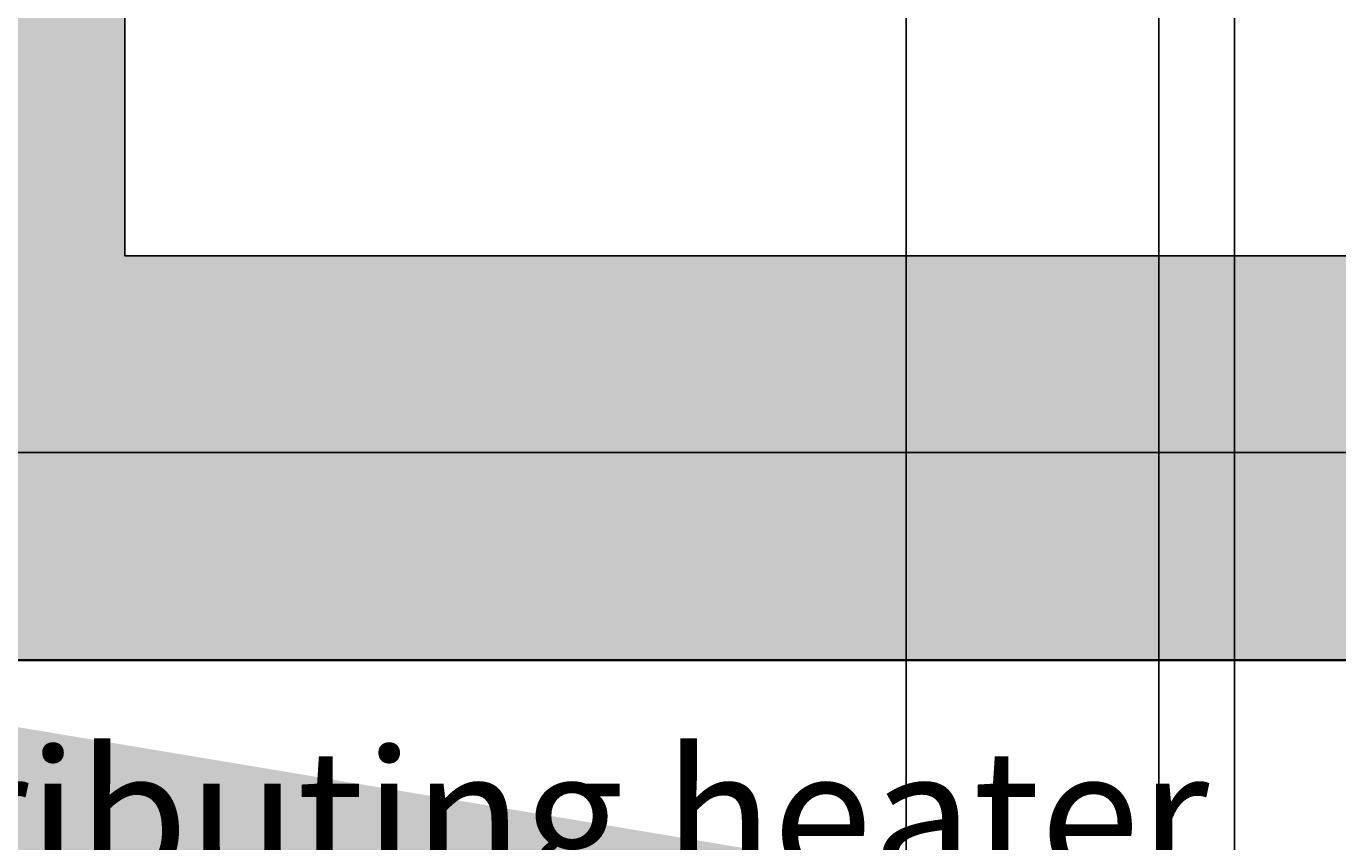
# Model space of a CAD drawing. Units: millimetres. Extents: x -22994 to 29398, y -19990 to 20176.
# Tile 27 of 135: x 99 to 139, y 5 to 30. Entities that reach past the tile are written whole.
import ezdxf
from ezdxf import colors
from ezdxf.entities.mleader import LeaderData, LeaderLine
from ezdxf.math import Vec2, Vec3

# ---------------------------------------------------------------- set-up
doc = ezdxf.new("R2010")
doc.units = ezdxf.units.MM
doc.header["$MEASUREMENT"] = 0
for name, color, linetype, lineweight in [('M-ANNO-TEXT', 7, 'Continuous', 25), ('M-DIMS', 2, 'Continuous', 18), ('M-EQPM', 7, 'Continuous', 25), ('M-EQPM-PATT', 7, 'Continuous', 18), ('S-FNDN', 7, 'Continuous', 35)]:
    doc.layers.add(name, color=color, linetype=linetype, lineweight=lineweight)
doc.styles.get("Standard").update_dxf_attribs({"font": 'arial.ttf'})
doc.dimstyles.get("Standard").update_dxf_attribs({"dimtxt": 0.18, "dimasz": 10000, "dimexe": 0.18, "dimexo": 0.0625, "dimgap": 0.09, "dimtad": 0, "dimtih": 1, "dimtoh": 1, "dimdec": 0, "dimzin": 0, "dimdsep": 46, "dimtxsty": 'Standard', "dimcen": 0.09, "dimadec": 0, "dimazin": 0, "dimtfac": 1, "dimtdec": 0, "dimtofl": 0, "dimtmove": 0, "dimatfit": 3, "dimfxl": 1, "dimtolj": 1, "dimtzin": 0, "dimlwd": 30, "dimarcsym": 0})

# ---------------------------------------------------------------- blocks, each defined once
blk = doc.blocks.new('*D2')
at = {"layer": 'Defpoints', "color": 0, "transparency": 16777216}
for p in [(6.677, 10.271), (290.852, 10.271), (290.852, -5.079)]:
    blk.add_point(p, dxfattribs=at)
at = {"layer": 'M-DIMS', "color": 0, "lineweight": -2, "transparency": 16777216}
for p, q in [((6.677, 10.209), (6.677, -5.259)), ((290.852, 10.209), (290.852, -5.259))]:
    blk.add_line(p, q, dxfattribs=at)
at = {"layer": 'M-DIMS', "color": 0, "lineweight": 30, "transparency": 16777216}
for p, q in [((-9993.323, -5.079), (-19993.323, -5.079)), ((10290.852, -5.079), (20290.852, -5.079))]:
    blk.add_line(p, q, dxfattribs=at)
at = {"layer": 'M-DIMS', "color": 0, "transparency": 16777216}
for points in [[(-9993.323, 1661.588), (-9993.323, -1671.745), (6.677, -5.079)], [(10290.852, 1661.588), (10290.852, -1671.745), (290.852, -5.079)]]:
    blk.add_solid(points, dxfattribs=at)
at = {"layer": 'M-DIMS', "color": 0, "transparency": 16777216, "insert": (148.765, -5.079), "char_height": 0.18, "attachment_point": 5}
blk.add_mtext('\\A1;284.2', dxfattribs=at)
blk = doc.blocks.new('*D3')
at = {"layer": 'Defpoints', "color": 0, "transparency": 16777216}
for p in [(110.265, 204.165), (110.265, 176.366), (95.833, 127.967)]:
    blk.add_point(p, dxfattribs=at)
at = {"layer": 'M-DIMS', "color": 0, "lineweight": -2, "transparency": 16777216}
for p, q in [((95.833, 128.03), (95.833, 204.345)), ((110.265, 176.429), (110.265, 204.345))]:
    blk.add_line(p, q, dxfattribs=at)
at = {"layer": 'M-DIMS', "color": 0, "lineweight": 30, "transparency": 16777216}
for p, q in [((-9904.167, 204.165), (-19904.167, 204.165)), ((10110.265, 204.165), (20110.265, 204.165))]:
    blk.add_line(p, q, dxfattribs=at)
at = {"layer": 'M-DIMS', "color": 0, "transparency": 16777216}
for points in [[(-9904.167, 1870.832), (-9904.167, -1462.501), (95.833, 204.165)], [(10110.265, 1870.832), (10110.265, -1462.501), (110.265, 204.165)]]:
    blk.add_solid(points, dxfattribs=at)
at = {"layer": 'M-DIMS', "color": 0, "transparency": 16777216, "insert": (103.049, 204.165), "char_height": 0.18, "attachment_point": 5}
blk.add_mtext('\\A1;14.432', dxfattribs=at)
blk = doc.blocks.new('*D4')
at = {"layer": 'Defpoints', "color": 0, "transparency": 16777216}
for p in [(116.265, 204.165), (110.265, 176.366), (116.265, 176.366)]:
    blk.add_point(p, dxfattribs=at)
at = {"layer": 'M-DIMS', "color": 0, "lineweight": -2, "transparency": 16777216}
for p, q in [((110.265, 176.429), (110.265, 204.345)), ((116.265, 176.429), (116.265, 204.345))]:
    blk.add_line(p, q, dxfattribs=at)
at = {"layer": 'M-DIMS', "color": 0, "lineweight": 30, "transparency": 16777216}
for p, q in [((-9889.735, 204.165), (-19889.735, 204.165)), ((10116.265, 204.165), (20116.265, 204.165))]:
    blk.add_line(p, q, dxfattribs=at)
at = {"layer": 'M-DIMS', "color": 0, "transparency": 16777216}
for points in [[(-9889.735, 1870.832), (-9889.735, -1462.501), (110.265, 204.165)], [(10116.265, 1870.832), (10116.265, -1462.501), (116.265, 204.165)]]:
    blk.add_solid(points, dxfattribs=at)
at = {"layer": 'M-DIMS', "color": 0, "transparency": 16777216, "insert": (113.265, 204.165), "char_height": 0.18, "attachment_point": 5}
blk.add_mtext('\\A1;6', dxfattribs=at)
blk = doc.blocks.new('*D5')
at = {"layer": 'Defpoints', "color": 0, "transparency": 16777216}
for p in [(181.265, 204.165), (116.265, 176.366), (181.265, 176.366)]:
    blk.add_point(p, dxfattribs=at)
at = {"layer": 'M-DIMS', "color": 0, "lineweight": -2, "transparency": 16777216}
for p, q in [((116.265, 176.429), (116.265, 204.345)), ((181.265, 176.429), (181.265, 204.345))]:
    blk.add_line(p, q, dxfattribs=at)
at = {"layer": 'M-DIMS', "color": 0, "lineweight": 30, "transparency": 16777216}
for p, q in [((-9883.735, 204.165), (-19883.735, 204.165)), ((10181.265, 204.165), (20181.265, 204.165))]:
    blk.add_line(p, q, dxfattribs=at)
at = {"layer": 'M-DIMS', "color": 0, "transparency": 16777216}
for points in [[(-9883.735, 1870.832), (-9883.735, -1462.501), (116.265, 204.165)], [(10181.265, 1870.832), (10181.265, -1462.501), (181.265, 204.165)]]:
    blk.add_solid(points, dxfattribs=at)
at = {"layer": 'M-DIMS', "color": 0, "transparency": 16777216, "insert": (148.765, 204.165), "char_height": 0.18, "attachment_point": 5}
blk.add_mtext('\\A1;65', dxfattribs=at)
blk = doc.blocks.new('*D6')
at = {"layer": 'Defpoints', "color": 0, "transparency": 16777216}
for p in [(187.265, 204.165), (181.265, 176.366), (187.265, 176.366)]:
    blk.add_point(p, dxfattribs=at)
at = {"layer": 'M-DIMS', "color": 0, "lineweight": -2, "transparency": 16777216}
for p, q in [((181.265, 176.429), (181.265, 204.345)), ((187.265, 176.429), (187.265, 204.345))]:
    blk.add_line(p, q, dxfattribs=at)
at = {"layer": 'M-DIMS', "color": 0, "lineweight": 30, "transparency": 16777216}
for p, q in [((-9818.735, 204.165), (-19818.735, 204.165)), ((10187.265, 204.165), (20187.265, 204.165))]:
    blk.add_line(p, q, dxfattribs=at)
at = {"layer": 'M-DIMS', "color": 0, "transparency": 16777216}
for points in [[(-9818.735, 1870.832), (-9818.735, -1462.501), (181.265, 204.165)], [(10187.265, 1870.832), (10187.265, -1462.501), (187.265, 204.165)]]:
    blk.add_solid(points, dxfattribs=at)
at = {"layer": 'M-DIMS', "color": 0, "transparency": 16777216, "insert": (184.265, 204.165), "char_height": 0.18, "attachment_point": 5}
blk.add_mtext('\\A1;6', dxfattribs=at)
blk = doc.blocks.new('*D7')
at = {"layer": 'Defpoints', "color": 0, "transparency": 16777216}
for p in [(201.697, 204.165), (187.265, 176.366), (201.697, 127.967)]:
    blk.add_point(p, dxfattribs=at)
at = {"layer": 'M-DIMS', "color": 0, "lineweight": -2, "transparency": 16777216}
for p, q in [((187.265, 176.429), (187.265, 204.345)), ((201.697, 128.03), (201.697, 204.345))]:
    blk.add_line(p, q, dxfattribs=at)
at = {"layer": 'M-DIMS', "color": 0, "lineweight": 30, "transparency": 16777216}
for p, q in [((-9812.735, 204.165), (-19812.735, 204.165)), ((10201.697, 204.165), (20201.697, 204.165))]:
    blk.add_line(p, q, dxfattribs=at)
at = {"layer": 'M-DIMS', "color": 0, "transparency": 16777216}
for points in [[(-9812.735, 1870.832), (-9812.735, -1462.501), (187.265, 204.165)], [(10201.697, 1870.832), (10201.697, -1462.501), (201.697, 204.165)]]:
    blk.add_solid(points, dxfattribs=at)
at = {"layer": 'M-DIMS', "color": 0, "transparency": 16777216, "insert": (194.481, 204.165), "char_height": 0.18, "attachment_point": 5}
blk.add_mtext('\\A1;14.432', dxfattribs=at)
blk = doc.blocks.new('*D8')
at = {"layer": 'Defpoints', "color": 0, "transparency": 16777216}
for p in [(227.648, 204.165), (227.648, 146.73), (201.697, 127.967)]:
    blk.add_point(p, dxfattribs=at)
at = {"layer": 'M-DIMS', "color": 0, "lineweight": -2, "transparency": 16777216}
for p, q in [((201.697, 128.03), (201.697, 204.345)), ((227.648, 146.792), (227.648, 204.345))]:
    blk.add_line(p, q, dxfattribs=at)
at = {"layer": 'M-DIMS', "color": 0, "lineweight": 30, "transparency": 16777216}
for p, q in [((-9798.303, 204.165), (-19798.303, 204.165)), ((10227.648, 204.165), (20227.648, 204.165))]:
    blk.add_line(p, q, dxfattribs=at)
at = {"layer": 'M-DIMS', "color": 0, "transparency": 16777216}
for points in [[(-9798.303, 1870.832), (-9798.303, -1462.501), (201.697, 204.165)], [(10227.648, 1870.832), (10227.648, -1462.501), (227.648, 204.165)]]:
    blk.add_solid(points, dxfattribs=at)
at = {"layer": 'M-DIMS', "color": 0, "transparency": 16777216, "insert": (214.673, 204.165), "char_height": 0.18, "attachment_point": 5}
blk.add_mtext('\\A1;25.95', dxfattribs=at)
blk = doc.blocks.new('*D9')
at = {"layer": 'Defpoints', "color": 0, "transparency": 16777216}
for p in [(187.265, 176.366), (306.202, 176.366), (290.852, 10.271)]:
    blk.add_point(p, dxfattribs=at)
at = {"layer": 'M-DIMS', "color": 0, "lineweight": 30, "transparency": 16777216}
for p, q in [((306.202, 10176.366), (306.202, 20176.366)), ((306.202, -9989.729), (306.202, -19989.729))]:
    blk.add_line(p, q, dxfattribs=at)
at = {"layer": 'M-DIMS', "color": 0, "lineweight": -2, "transparency": 16777216}
for p, q in [((187.327, 176.366), (306.382, 176.366)), ((290.915, 10.271), (306.382, 10.271))]:
    blk.add_line(p, q, dxfattribs=at)
at = {"layer": 'M-DIMS', "color": 0, "transparency": 16777216}
for points in [[(-1360.465, 10176.366), (1972.869, 10176.366), (306.202, 176.366)], [(-1360.465, -9989.729), (1972.869, -9989.729), (306.202, 10.271)]]:
    blk.add_solid(points, dxfattribs=at)
at = {"layer": 'M-DIMS', "color": 0, "transparency": 16777216, "insert": (306.202, 93.319), "char_height": 0.18, "attachment_point": 5}
blk.add_mtext('\\A1;166.1', dxfattribs=at)
blk = doc.blocks.new('*D10')
at = {"layer": 'Defpoints', "color": 0, "transparency": 16777216}
for p in [(125.65, 136.071), (133.346, 136.071), (133.346, -5.079)]:
    blk.add_point(p, dxfattribs=at)
at = {"layer": 'M-DIMS', "color": 0, "lineweight": -2, "transparency": 16777216}
for p, q in [((125.65, 136.009), (125.65, -5.259)), ((133.346, 136.009), (133.346, -5.259))]:
    blk.add_line(p, q, dxfattribs=at)
at = {"layer": 'M-DIMS', "color": 0, "lineweight": 30, "transparency": 16777216}
for p, q in [((-9874.35, -5.079), (-19874.35, -5.079)), ((10133.346, -5.079), (20133.346, -5.079))]:
    blk.add_line(p, q, dxfattribs=at)
at = {"layer": 'M-DIMS', "color": 0, "transparency": 16777216}
for points in [[(-9874.35, 1661.588), (-9874.35, -1671.745), (125.65, -5.079)], [(10133.346, 1661.588), (10133.346, -1671.745), (133.346, -5.079)]]:
    blk.add_solid(points, dxfattribs=at)
at = {"layer": 'M-DIMS', "color": 0, "transparency": 16777216, "insert": (129.498, -5.079), "char_height": 0.18, "attachment_point": 5}
blk.add_mtext('\\A1;7.696', dxfattribs=at)
blk = doc.blocks.new('*D11')
at = {"layer": 'Defpoints', "color": 0, "transparency": 16777216}
for p in [(133.346, 136.071), (135.65, 136.071), (135.65, -5.079)]:
    blk.add_point(p, dxfattribs=at)
at = {"layer": 'M-DIMS', "color": 0, "lineweight": -2, "transparency": 16777216}
for p, q in [((133.346, 136.009), (133.346, -5.259)), ((135.65, 136.009), (135.65, -5.259))]:
    blk.add_line(p, q, dxfattribs=at)
at = {"layer": 'M-DIMS', "color": 0, "lineweight": 30, "transparency": 16777216}
for p, q in [((-9866.654, -5.079), (-19866.654, -5.079)), ((10135.65, -5.079), (20135.65, -5.079))]:
    blk.add_line(p, q, dxfattribs=at)
at = {"layer": 'M-DIMS', "color": 0, "transparency": 16777216}
for points in [[(-9866.654, 1661.588), (-9866.654, -1671.745), (133.346, -5.079)], [(10135.65, 1661.588), (10135.65, -1671.745), (135.65, -5.079)]]:
    blk.add_solid(points, dxfattribs=at)
at = {"layer": 'M-DIMS', "color": 0, "transparency": 16777216, "insert": (134.498, -5.079), "char_height": 0.18, "attachment_point": 5}
blk.add_mtext('\\A1;2.304', dxfattribs=at)
blk = doc.blocks.new('*D12')
at = {"layer": 'Defpoints', "color": 0, "transparency": 16777216}
for p in [(135.65, 136.071), (145.65, 136.071), (145.65, -5.079)]:
    blk.add_point(p, dxfattribs=at)
at = {"layer": 'M-DIMS', "color": 0, "lineweight": -2, "transparency": 16777216}
for p, q in [((135.65, 136.009), (135.65, -5.259)), ((145.65, 136.009), (145.65, -5.259))]:
    blk.add_line(p, q, dxfattribs=at)
at = {"layer": 'M-DIMS', "color": 0, "lineweight": 30, "transparency": 16777216}
for p, q in [((-9864.35, -5.079), (-19864.35, -5.079)), ((10145.65, -5.079), (20145.65, -5.079))]:
    blk.add_line(p, q, dxfattribs=at)
at = {"layer": 'M-DIMS', "color": 0, "transparency": 16777216}
for points in [[(-9864.35, 1661.588), (-9864.35, -1671.745), (135.65, -5.079)], [(10145.65, 1661.588), (10145.65, -1671.745), (145.65, -5.079)]]:
    blk.add_solid(points, dxfattribs=at)
at = {"layer": 'M-DIMS', "color": 0, "transparency": 16777216, "insert": (140.65, -5.079), "char_height": 0.18, "attachment_point": 5}
blk.add_mtext('\\A1;10', dxfattribs=at)
blk = doc.blocks.new('*D13')
at = {"layer": 'Defpoints', "color": 0, "transparency": 16777216}
for p in [(145.65, 136.071), (155.65, 136.071), (155.65, -5.079)]:
    blk.add_point(p, dxfattribs=at)
at = {"layer": 'M-DIMS', "color": 0, "lineweight": -2, "transparency": 16777216}
for p, q in [((145.65, 136.009), (145.65, -5.259)), ((155.65, 136.009), (155.65, -5.259))]:
    blk.add_line(p, q, dxfattribs=at)
at = {"layer": 'M-DIMS', "color": 0, "lineweight": 30, "transparency": 16777216}
for p, q in [((-9854.35, -5.079), (-19854.35, -5.079)), ((10155.65, -5.079), (20155.65, -5.079))]:
    blk.add_line(p, q, dxfattribs=at)
at = {"layer": 'M-DIMS', "color": 0, "transparency": 16777216}
for points in [[(-9854.35, 1661.588), (-9854.35, -1671.745), (145.65, -5.079)], [(10155.65, 1661.588), (10155.65, -1671.745), (155.65, -5.079)]]:
    blk.add_solid(points, dxfattribs=at)
at = {"layer": 'M-DIMS', "color": 0, "transparency": 16777216, "insert": (150.65, -5.079), "char_height": 0.18, "attachment_point": 5}
blk.add_mtext('\\A1;10', dxfattribs=at)
blk = doc.blocks.new('*D14')
at = {"layer": 'Defpoints', "color": 0, "transparency": 16777216}
for p in [(155.65, 136.071), (165.65, 136.071), (165.65, -5.079)]:
    blk.add_point(p, dxfattribs=at)
at = {"layer": 'M-DIMS', "color": 0, "lineweight": -2, "transparency": 16777216}
for p, q in [((155.65, 136.009), (155.65, -5.259)), ((165.65, 136.009), (165.65, -5.259))]:
    blk.add_line(p, q, dxfattribs=at)
at = {"layer": 'M-DIMS', "color": 0, "lineweight": 30, "transparency": 16777216}
for p, q in [((-9844.35, -5.079), (-19844.35, -5.079)), ((10165.65, -5.079), (20165.65, -5.079))]:
    blk.add_line(p, q, dxfattribs=at)
at = {"layer": 'M-DIMS', "color": 0, "transparency": 16777216}
for points in [[(-9844.35, 1661.588), (-9844.35, -1671.745), (155.65, -5.079)], [(10165.65, 1661.588), (10165.65, -1671.745), (165.65, -5.079)]]:
    blk.add_solid(points, dxfattribs=at)
at = {"layer": 'M-DIMS', "color": 0, "transparency": 16777216, "insert": (160.65, -5.079), "char_height": 0.18, "attachment_point": 5}
blk.add_mtext('\\A1;10', dxfattribs=at)
blk = doc.blocks.new('*D15')
at = {"layer": 'Defpoints', "color": 0, "transparency": 16777216}
for p in [(173.346, 154.788), (173.346, 136.071), (306.202, 136.071)]:
    blk.add_point(p, dxfattribs=at)
at = {"layer": 'M-DIMS', "color": 0, "lineweight": 30, "transparency": 16777216}
for p, q in [((306.202, 10154.788), (306.202, 20154.788)), ((306.202, -9863.929), (306.202, -19863.929))]:
    blk.add_line(p, q, dxfattribs=at)
at = {"layer": 'M-DIMS', "color": 0, "lineweight": -2, "transparency": 16777216}
for p, q in [((173.408, 154.788), (306.382, 154.788)), ((173.408, 136.071), (306.382, 136.071))]:
    blk.add_line(p, q, dxfattribs=at)
at = {"layer": 'M-DIMS', "color": 0, "transparency": 16777216}
for points in [[(-1360.465, 10154.788), (1972.869, 10154.788), (306.202, 154.788)], [(-1360.465, -9863.929), (1972.869, -9863.929), (306.202, 136.071)]]:
    blk.add_solid(points, dxfattribs=at)
at = {"layer": 'M-DIMS', "color": 0, "transparency": 16777216, "insert": (306.202, 145.43), "char_height": 0.18, "attachment_point": 5}
blk.add_mtext('\\A1;18.717', dxfattribs=at)
blk = doc.blocks.new('*D16')
at = {"layer": 'Defpoints', "color": 0, "transparency": 16777216}
for p in [(120.17, 204.165), (110.466, 48.035), (120.17, 48.035)]:
    blk.add_point(p, dxfattribs=at)
at = {"layer": 'M-DIMS', "color": 0, "lineweight": -2, "transparency": 16777216}
for p, q in [((110.466, 48.097), (110.466, 204.345)), ((120.17, 48.097), (120.17, 204.345))]:
    blk.add_line(p, q, dxfattribs=at)
at = {"layer": 'M-DIMS', "color": 0, "lineweight": 30, "transparency": 16777216}
for p, q in [((-9889.534, 204.165), (-19889.534, 204.165)), ((10120.17, 204.165), (20120.17, 204.165))]:
    blk.add_line(p, q, dxfattribs=at)
at = {"layer": 'M-DIMS', "color": 0, "transparency": 16777216}
for points in [[(-9889.534, 1870.832), (-9889.534, -1462.501), (110.466, 204.165)], [(10120.17, 1870.832), (10120.17, -1462.501), (120.17, 204.165)]]:
    blk.add_solid(points, dxfattribs=at)
at = {"layer": 'M-DIMS', "color": 0, "transparency": 16777216, "insert": (115.318, 204.165), "char_height": 0.18, "attachment_point": 5}
blk.add_mtext('\\A1;9.704', dxfattribs=at)
blk = doc.blocks.new('*D17')
at = {"layer": 'Defpoints', "color": 0, "transparency": 16777216}
for p in [(126.17, 204.165), (120.17, 48.035), (126.17, 48.035)]:
    blk.add_point(p, dxfattribs=at)
at = {"layer": 'M-DIMS', "color": 0, "lineweight": -2, "transparency": 16777216}
for p, q in [((120.17, 48.097), (120.17, 204.345)), ((126.17, 48.097), (126.17, 204.345))]:
    blk.add_line(p, q, dxfattribs=at)
at = {"layer": 'M-DIMS', "color": 0, "lineweight": 30, "transparency": 16777216}
for p, q in [((-9879.83, 204.165), (-19879.83, 204.165)), ((10126.17, 204.165), (20126.17, 204.165))]:
    blk.add_line(p, q, dxfattribs=at)
at = {"layer": 'M-DIMS', "color": 0, "transparency": 16777216}
for points in [[(-9879.83, 1870.832), (-9879.83, -1462.501), (120.17, 204.165)], [(10126.17, 1870.832), (10126.17, -1462.501), (126.17, 204.165)]]:
    blk.add_solid(points, dxfattribs=at)
at = {"layer": 'M-DIMS', "color": 0, "transparency": 16777216, "insert": (123.17, 204.165), "char_height": 0.18, "attachment_point": 5}
blk.add_mtext('\\A1;6', dxfattribs=at)
blk = doc.blocks.new('*D18')
at = {"layer": 'Defpoints', "color": 0, "transparency": 16777216}
for p in [(132.17, 204.165), (126.17, 48.035), (132.17, 48.035)]:
    blk.add_point(p, dxfattribs=at)
at = {"layer": 'M-DIMS', "color": 0, "lineweight": -2, "transparency": 16777216}
for p, q in [((126.17, 48.097), (126.17, 204.345)), ((132.17, 48.097), (132.17, 204.345))]:
    blk.add_line(p, q, dxfattribs=at)
at = {"layer": 'M-DIMS', "color": 0, "lineweight": 30, "transparency": 16777216}
for p, q in [((-9873.83, 204.165), (-19873.83, 204.165)), ((10132.17, 204.165), (20132.17, 204.165))]:
    blk.add_line(p, q, dxfattribs=at)
at = {"layer": 'M-DIMS', "color": 0, "transparency": 16777216}
for points in [[(-9873.83, 1870.832), (-9873.83, -1462.501), (126.17, 204.165)], [(10132.17, 1870.832), (10132.17, -1462.501), (132.17, 204.165)]]:
    blk.add_solid(points, dxfattribs=at)
at = {"layer": 'M-DIMS', "color": 0, "transparency": 16777216, "insert": (129.17, 204.165), "char_height": 0.18, "attachment_point": 5}
blk.add_mtext('\\A1;6', dxfattribs=at)
blk = doc.blocks.new('*D19')
at = {"layer": 'Defpoints', "color": 0, "transparency": 16777216}
for p in [(138.17, 204.165), (132.17, 48.035), (138.17, 48.035)]:
    blk.add_point(p, dxfattribs=at)
at = {"layer": 'M-DIMS', "color": 0, "lineweight": -2, "transparency": 16777216}
for p, q in [((132.17, 48.097), (132.17, 204.345)), ((138.17, 48.097), (138.17, 204.345))]:
    blk.add_line(p, q, dxfattribs=at)
at = {"layer": 'M-DIMS', "color": 0, "lineweight": 30, "transparency": 16777216}
for p, q in [((-9867.83, 204.165), (-19867.83, 204.165)), ((10138.17, 204.165), (20138.17, 204.165))]:
    blk.add_line(p, q, dxfattribs=at)
at = {"layer": 'M-DIMS', "color": 0, "transparency": 16777216}
for points in [[(-9867.83, 1870.832), (-9867.83, -1462.501), (132.17, 204.165)], [(10138.17, 1870.832), (10138.17, -1462.501), (138.17, 204.165)]]:
    blk.add_solid(points, dxfattribs=at)
at = {"layer": 'M-DIMS', "color": 0, "transparency": 16777216, "insert": (135.17, 204.165), "char_height": 0.18, "attachment_point": 5}
blk.add_mtext('\\A1;6', dxfattribs=at)
blk = doc.blocks.new('*D20')
at = {"layer": 'Defpoints', "color": 0, "transparency": 16777216}
for p in [(144.17, 204.165), (138.17, 48.035), (144.17, 48.035)]:
    blk.add_point(p, dxfattribs=at)
at = {"layer": 'M-DIMS', "color": 0, "lineweight": -2, "transparency": 16777216}
for p, q in [((138.17, 48.097), (138.17, 204.345)), ((144.17, 48.097), (144.17, 204.345))]:
    blk.add_line(p, q, dxfattribs=at)
at = {"layer": 'M-DIMS', "color": 0, "lineweight": 30, "transparency": 16777216}
for p, q in [((-9861.83, 204.165), (-19861.83, 204.165)), ((10144.17, 204.165), (20144.17, 204.165))]:
    blk.add_line(p, q, dxfattribs=at)
at = {"layer": 'M-DIMS', "color": 0, "transparency": 16777216}
for points in [[(-9861.83, 1870.832), (-9861.83, -1462.501), (138.17, 204.165)], [(10144.17, 1870.832), (10144.17, -1462.501), (144.17, 204.165)]]:
    blk.add_solid(points, dxfattribs=at)
at = {"layer": 'M-DIMS', "color": 0, "transparency": 16777216, "insert": (141.17, 204.165), "char_height": 0.18, "attachment_point": 5}
blk.add_mtext('\\A1;6', dxfattribs=at)
blk = doc.blocks.new('*D21')
at = {"layer": 'Defpoints', "color": 0, "transparency": 16777216}
for p in [(149.116, 204.165), (144.17, 48.035), (149.116, 48.035)]:
    blk.add_point(p, dxfattribs=at)
at = {"layer": 'M-DIMS', "color": 0, "lineweight": -2, "transparency": 16777216}
for p, q in [((144.17, 48.097), (144.17, 204.345)), ((149.116, 48.097), (149.116, 204.345))]:
    blk.add_line(p, q, dxfattribs=at)
at = {"layer": 'M-DIMS', "color": 0, "lineweight": 30, "transparency": 16777216}
for p, q in [((-9855.83, 204.165), (-19855.83, 204.165)), ((10149.116, 204.165), (20149.116, 204.165))]:
    blk.add_line(p, q, dxfattribs=at)
at = {"layer": 'M-DIMS', "color": 0, "transparency": 16777216}
for points in [[(-9855.83, 1870.832), (-9855.83, -1462.501), (144.17, 204.165)], [(10149.116, 1870.832), (10149.116, -1462.501), (149.116, 204.165)]]:
    blk.add_solid(points, dxfattribs=at)
at = {"layer": 'M-DIMS', "color": 0, "transparency": 16777216, "insert": (146.643, 204.165), "char_height": 0.18, "attachment_point": 5}
blk.add_mtext('\\A1;4.945', dxfattribs=at)
blk = doc.blocks.new('*D22')
at = {"layer": 'Defpoints', "color": 0, "transparency": 16777216}
for p in [(149.116, 30.99), (155.116, 30.99), (155.116, -5.079)]:
    blk.add_point(p, dxfattribs=at)
at = {"layer": 'M-DIMS', "color": 0, "lineweight": -2, "transparency": 16777216}
for p, q in [((149.116, 30.927), (149.116, -5.259)), ((155.116, 30.927), (155.116, -5.259))]:
    blk.add_line(p, q, dxfattribs=at)
at = {"layer": 'M-DIMS', "color": 0, "lineweight": 30, "transparency": 16777216}
for p, q in [((-9850.884, -5.079), (-19850.884, -5.079)), ((10155.116, -5.079), (20155.116, -5.079))]:
    blk.add_line(p, q, dxfattribs=at)
at = {"layer": 'M-DIMS', "color": 0, "transparency": 16777216}
for points in [[(-9850.884, 1661.588), (-9850.884, -1671.745), (149.116, -5.079)], [(10155.116, 1661.588), (10155.116, -1671.745), (155.116, -5.079)]]:
    blk.add_solid(points, dxfattribs=at)
at = {"layer": 'M-DIMS', "color": 0, "transparency": 16777216, "insert": (152.116, -5.079), "char_height": 0.18, "attachment_point": 5}
blk.add_mtext('\\A1;6', dxfattribs=at)
blk = doc.blocks.new('*D23')
at = {"layer": 'Defpoints', "color": 0, "transparency": 16777216}
for p in [(155.116, 30.99), (161.116, 30.99), (161.116, -5.079)]:
    blk.add_point(p, dxfattribs=at)
at = {"layer": 'M-DIMS', "color": 0, "lineweight": -2, "transparency": 16777216}
for p, q in [((155.116, 30.927), (155.116, -5.259)), ((161.116, 30.927), (161.116, -5.259))]:
    blk.add_line(p, q, dxfattribs=at)
at = {"layer": 'M-DIMS', "color": 0, "lineweight": 30, "transparency": 16777216}
for p, q in [((-9844.884, -5.079), (-19844.884, -5.079)), ((10161.116, -5.079), (20161.116, -5.079))]:
    blk.add_line(p, q, dxfattribs=at)
at = {"layer": 'M-DIMS', "color": 0, "transparency": 16777216}
for points in [[(-9844.884, 1661.588), (-9844.884, -1671.745), (155.116, -5.079)], [(10161.116, 1661.588), (10161.116, -1671.745), (161.116, -5.079)]]:
    blk.add_solid(points, dxfattribs=at)
at = {"layer": 'M-DIMS', "color": 0, "transparency": 16777216, "insert": (158.116, -5.079), "char_height": 0.18, "attachment_point": 5}
blk.add_mtext('\\A1;6', dxfattribs=at)
blk = doc.blocks.new('*D24')
at = {"layer": 'Defpoints', "color": 0, "transparency": 16777216}
for p in [(161.116, 30.99), (166.439, 30.99), (166.439, -5.079)]:
    blk.add_point(p, dxfattribs=at)
at = {"layer": 'M-DIMS', "color": 0, "lineweight": -2, "transparency": 16777216}
for p, q in [((161.116, 30.927), (161.116, -5.259)), ((166.439, 30.927), (166.439, -5.259))]:
    blk.add_line(p, q, dxfattribs=at)
at = {"layer": 'M-DIMS', "color": 0, "lineweight": 30, "transparency": 16777216}
for p, q in [((-9838.884, -5.079), (-19838.884, -5.079)), ((10166.439, -5.079), (20166.439, -5.079))]:
    blk.add_line(p, q, dxfattribs=at)
at = {"layer": 'M-DIMS', "color": 0, "transparency": 16777216}
for points in [[(-9838.884, 1661.588), (-9838.884, -1671.745), (161.116, -5.079)], [(10166.439, 1661.588), (10166.439, -1671.745), (166.439, -5.079)]]:
    blk.add_solid(points, dxfattribs=at)
at = {"layer": 'M-DIMS', "color": 0, "transparency": 16777216, "insert": (163.777, -5.079), "char_height": 0.18, "attachment_point": 5}
blk.add_mtext('\\A1;5.323', dxfattribs=at)
blk = doc.blocks.new('*D25')
at = {"layer": 'Defpoints', "color": 0, "transparency": 16777216}
for p in [(166.439, 30.99), (172.439, 30.99), (172.439, -5.079)]:
    blk.add_point(p, dxfattribs=at)
at = {"layer": 'M-DIMS', "color": 0, "lineweight": -2, "transparency": 16777216}
for p, q in [((166.439, 30.927), (166.439, -5.259)), ((172.439, 30.927), (172.439, -5.259))]:
    blk.add_line(p, q, dxfattribs=at)
at = {"layer": 'M-DIMS', "color": 0, "lineweight": 30, "transparency": 16777216}
for p, q in [((-9833.561, -5.079), (-19833.561, -5.079)), ((10172.439, -5.079), (20172.439, -5.079))]:
    blk.add_line(p, q, dxfattribs=at)
at = {"layer": 'M-DIMS', "color": 0, "transparency": 16777216}
for points in [[(-9833.561, 1661.588), (-9833.561, -1671.745), (166.439, -5.079)], [(10172.439, 1661.588), (10172.439, -1671.745), (172.439, -5.079)]]:
    blk.add_solid(points, dxfattribs=at)
at = {"layer": 'M-DIMS', "color": 0, "transparency": 16777216, "insert": (169.439, -5.079), "char_height": 0.18, "attachment_point": 5}
blk.add_mtext('\\A1;6', dxfattribs=at)
blk = doc.blocks.new('*D26')
at = {"layer": 'Defpoints', "color": 0, "transparency": 16777216}
for p in [(172.439, 30.99), (178.439, 30.99), (178.439, -5.079)]:
    blk.add_point(p, dxfattribs=at)
at = {"layer": 'M-DIMS', "color": 0, "lineweight": -2, "transparency": 16777216}
for p, q in [((172.439, 30.927), (172.439, -5.259)), ((178.439, 30.927), (178.439, -5.259))]:
    blk.add_line(p, q, dxfattribs=at)
at = {"layer": 'M-DIMS', "color": 0, "lineweight": 30, "transparency": 16777216}
for p, q in [((-9827.561, -5.079), (-19827.561, -5.079)), ((10178.439, -5.079), (20178.439, -5.079))]:
    blk.add_line(p, q, dxfattribs=at)
at = {"layer": 'M-DIMS', "color": 0, "transparency": 16777216}
for points in [[(-9827.561, 1661.588), (-9827.561, -1671.745), (172.439, -5.079)], [(10178.439, 1661.588), (10178.439, -1671.745), (178.439, -5.079)]]:
    blk.add_solid(points, dxfattribs=at)
at = {"layer": 'M-DIMS', "color": 0, "transparency": 16777216, "insert": (175.439, -5.079), "char_height": 0.18, "attachment_point": 5}
blk.add_mtext('\\A1;6', dxfattribs=at)
blk = doc.blocks.new('*D27')
at = {"layer": 'Defpoints', "color": 0, "transparency": 16777216}
for p in [(178.439, 30.99), (188.117, 30.99), (188.117, -5.079)]:
    blk.add_point(p, dxfattribs=at)
at = {"layer": 'M-DIMS', "color": 0, "lineweight": -2, "transparency": 16777216}
for p, q in [((178.439, 30.927), (178.439, -5.259)), ((188.117, 30.927), (188.117, -5.259))]:
    blk.add_line(p, q, dxfattribs=at)
at = {"layer": 'M-DIMS', "color": 0, "lineweight": 30, "transparency": 16777216}
for p, q in [((-9821.561, -5.079), (-19821.561, -5.079)), ((10188.117, -5.079), (20188.117, -5.079))]:
    blk.add_line(p, q, dxfattribs=at)
at = {"layer": 'M-DIMS', "color": 0, "transparency": 16777216}
for points in [[(-9821.561, 1661.588), (-9821.561, -1671.745), (178.439, -5.079)], [(10188.117, 1661.588), (10188.117, -1671.745), (188.117, -5.079)]]:
    blk.add_solid(points, dxfattribs=at)
at = {"layer": 'M-DIMS', "color": 0, "transparency": 16777216, "insert": (183.278, -5.079), "char_height": 0.18, "attachment_point": 5}
blk.add_mtext('\\A1;9.679', dxfattribs=at)
blk = doc.blocks.new('*D28')
at = {"layer": 'Defpoints', "color": 0, "transparency": 16777216}
for p in [(188.117, 48.035), (306.202, 48.035), (188.117, 30.99)]:
    blk.add_point(p, dxfattribs=at)
at = {"layer": 'M-DIMS', "color": 0, "lineweight": 30, "transparency": 16777216}
for p, q in [((306.202, 10048.035), (306.202, 20048.035)), ((306.202, -9969.01), (306.202, -19969.01))]:
    blk.add_line(p, q, dxfattribs=at)
at = {"layer": 'M-DIMS', "color": 0, "lineweight": -2, "transparency": 16777216}
for p, q in [((188.18, 48.035), (306.382, 48.035)), ((188.18, 30.99), (306.382, 30.99))]:
    blk.add_line(p, q, dxfattribs=at)
at = {"layer": 'M-DIMS', "color": 0, "transparency": 16777216}
for points in [[(-1360.465, 10048.035), (1972.869, 10048.035), (306.202, 48.035)], [(-1360.465, -9969.01), (1972.869, -9969.01), (306.202, 30.99)]]:
    blk.add_solid(points, dxfattribs=at)
at = {"layer": 'M-DIMS', "color": 0, "transparency": 16777216, "insert": (306.202, 39.512), "char_height": 0.18, "attachment_point": 5}
blk.add_mtext('\\A1;17.045', dxfattribs=at)
blk = doc.blocks.new('*D29')
at = {"layer": 'Defpoints', "color": 0, "transparency": 16777216}
for p in [(36.801, 80.045), (64.03, 80.045)]:
    blk.add_point(p, dxfattribs=at)
at = {"layer": 'M-DIMS', "color": 0, "lineweight": -2, "transparency": 16777216}
for p, q in [((50.325, 80.045), (50.505, 80.045)), ((50.415, 79.955), (50.415, 80.135))]:
    blk.add_line(p, q, dxfattribs=at)
at = {"layer": 'M-DIMS', "color": 0, "lineweight": 30, "transparency": 16777216}
blk.add_line((20064.03, 80.03), (10064.03, 80.038), dxfattribs=at)
at = {"layer": 'M-DIMS', "color": 0, "transparency": 16777216}
blk.add_solid([(10064.031, 1746.704), (10064.028, -1586.629), (64.03, 80.045)], dxfattribs=at)
at = {"layer": 'M-DIMS', "color": 0, "transparency": 16777216, "insert": (20064.521, 80.03), "char_height": 0.18, "attachment_point": 5}
blk.add_mtext('\\A1;∅27.23', dxfattribs=at)
blk = doc.blocks.new('*D36')
at = {"layer": 'Defpoints', "color": 0, "transparency": 16777216}
for p in [(46.39, 31.303), (46.387, 26.593)]:
    blk.add_point(p, dxfattribs=at)
at = {"layer": 'M-DIMS', "color": 0, "lineweight": 30, "transparency": 16777216}
for p, q in [((57.15, 20031.301), (51.77, 10031.302)), ((10057.15, 20031.301), (57.15, 20031.301))]:
    blk.add_line(p, q, dxfattribs=at)
at = {"layer": 'M-DIMS', "color": 0, "lineweight": -2, "transparency": 16777216}
for p, q in [((46.299, 28.948), (46.479, 28.948)), ((46.389, 28.858), (46.389, 29.038))]:
    blk.add_line(p, q, dxfattribs=at)
at = {"layer": 'M-DIMS', "color": 0, "transparency": 16777216}
blk.add_solid([(-1614.896, 10032.199), (1718.436, 10030.405), (46.39, 31.303)], dxfattribs=at)
at = {"layer": 'M-DIMS', "color": 0, "transparency": 16777216, "insert": (10057.554, 20031.301), "char_height": 0.18, "attachment_point": 5}
blk.add_mtext('\\A1;∅4.71', dxfattribs=at)
blk = doc.blocks.new('*D37')
at = {"layer": 'Defpoints', "color": 0, "transparency": 16777216}
for p in [(54.834, 118.615), (59.494, 118.614)]:
    blk.add_point(p, dxfattribs=at)
at = {"layer": 'M-DIMS', "color": 0, "lineweight": -2, "transparency": 16777216}
for p, q in [((57.164, 118.524), (57.164, 118.704)), ((57.074, 118.614), (57.254, 118.614))]:
    blk.add_line(p, q, dxfattribs=at)
at = {"layer": 'M-DIMS', "color": 0, "lineweight": 30, "transparency": 16777216}
blk.add_line((20059.493, 116.253), (10059.494, 117.434), dxfattribs=at)
at = {"layer": 'M-DIMS', "color": 0, "transparency": 16777216}
blk.add_solid([(10059.69, 1784.1), (10059.297, -1549.233), (59.494, 118.614)], dxfattribs=at)
at = {"layer": 'M-DIMS', "color": 0, "transparency": 16777216, "insert": (20059.985, 116.253), "char_height": 0.18, "attachment_point": 5}
blk.add_mtext('\\A1;∅4.659', dxfattribs=at)

msp = doc.modelspace()

# ---------------------------------------------------------------- hatches: boundary and pattern name
at = {"layer": 'M-EQPM-PATT'}
h = msp.add_hatch(color=256, dxfattribs=at)
h.set_gradient(color1=(205, 32, 39), color2=(205, 32, 39), tint=1)
h.paths.add_polyline_path([(116.2647, 150.3662), (116.2647, 170.3662), (116.2647, 176.3662), (110.2647, 176.3662), (110.2647, 152.0276), (95.8327, 127.967), (95.8327, 16.6063), (201.6967, 16.6063), (201.6967, 127.967), (187.2647, 152.0276), (187.2647, 176.3662), (181.2647, 176.3662), (181.2647, 170.3662), (181.2647, 150.3662), (195.6967, 126.3055), (195.6967, 22.6063), (101.8327, 22.6063), (101.8327, 126.3055)])
h.paths.add_polyline_path([(185.2208, 88.6347), (101.8327, 88.6347), (101.8327, 87.6347), (182.8066, 87.6347), (178.7313, 83.5594), (195.6967, 83.5594), (195.6967, 84.5594), (181.1455, 84.5594)], flags=17)
h.paths.add_polyline_path([(95.8327, 88.6347), (60.9779, 88.6347, -0.0228552), (61.7178, 87.6347), (95.8327, 87.6347)])
h.paths.add_polyline_path([(215.6212, 86.5189), (215.6212, 80.5999), (220.5095, 83.5594)])
h.paths.add_polyline_path([(215.6212, 84.5594), (201.6967, 84.5594), (201.6967, 83.5594), (215.6212, 83.5594)])
h.paths.add_polyline_path([(225.3978, 86.5189), (220.5095, 83.5594), (225.3978, 80.5999)])
h.paths.add_polyline_path([(231.6256, 84.5594), (225.3978, 84.5594), (225.3978, 83.5594), (231.6256, 83.5594)])
at = {"layer": 'S-FNDN'}
h = msp.add_hatch(color=256, dxfattribs=at)
h.set_gradient(color1=(241, 235, 31), color2=(244, 238, 81), tint=1, name='CYLINDER')
h.paths.add_polyline_path([(290.852, 16.6063), (201.6967, 16.6063), (95.8327, 16.6063), (81.8485, 16.6063), (82.3691, 10.2713), (290.852, 10.2713)])
h.paths.add_polyline_path([(81.8485, 16.6063), (60.8206, 16.6063), (62.0909, 10.2713), (82.3691, 10.2713)])
h.paths.add_polyline_path([(60.8206, 16.6063), (6.6773, 16.6063), (6.6773, 10.2713), (62.0909, 10.2713)])

# ---------------------------------------------------------------- linework, layer by layer
at = {"layer": 'M-EQPM'}
msp.add_lwpolyline([(110.2647, 176.3662), (110.2647, 152.0276), (95.8327, 127.967), (95.8327, 16.6063), (201.6967, 16.6063), (201.6967, 127.967), (187.2647, 152.0276), (187.2647, 176.3662)], close=True, dxfattribs=at)
msp.add_lwpolyline([(116.2647, 170.3662), (116.2647, 150.3662), (101.8327, 126.3055), (101.8327, 22.6063), (195.6967, 22.6063), (195.6967, 126.3055), (181.2647, 150.3662), (181.2647, 170.3662)], dxfattribs=at)
at = {"layer": 'S-FNDN'}
msp.add_lwpolyline([(95.8327, 16.6063), (6.6773, 16.6063), (6.6773, 10.2713), (290.852, 10.2713), (290.852, 16.6063), (201.6967, 16.6063)], dxfattribs=at)

# ---------------------------------------------------------------- dimensions: what is measured, and where the dimension line sits
at = {"layer": 'M-DIMS'}
for base, p1, p2, override, picture, middle in [((306.202, 176.3662), (290.852, 10.2713), (187.2647, 176.3662), {"dimdec": 1, "dimlfac": 1, "dimrnd": 0, "dimzin": 0, "dimdsep": 46, "dimlunit": 2}, '*D9', (306.202, 93.3187)), ((306.202, 136.0713), (173.3459, 154.788), (173.3459, 136.0713), {"dimdec": 3, "dimlfac": 1, "dimrnd": 0, "dimzin": 0, "dimdsep": 46, "dimlunit": 2}, '*D15', (306.202, 145.4297)), ((306.202, 48.0349), (188.1175, 30.9895), (188.1175, 48.0349), {"dimdec": 3, "dimlfac": 1, "dimrnd": 0, "dimzin": 0, "dimdsep": 46, "dimlunit": 2}, '*D28', (306.202, 39.5122))]:
    dim = msp.add_linear_dim(base=base, p1=p1, p2=p2, angle=90, dimstyle='Standard', override=override, dxfattribs=at)
    dim.commit()
    dim.dimension.update_dxf_attribs({"geometry": picture, "text_midpoint": middle})
dim = msp.add_diameter_dim_2p(p1=(46.3875, 26.5934), p2=(46.39, 31.3035), dimstyle='Standard', override={"dimdec": 2, "dimlfac": 1, "dimrnd": 0, "dimzin": 0, "dimdsep": 46, "dimlunit": 2}, dxfattribs=at)
dim.commit()
dim.dimension.update_dxf_attribs({"geometry": '*D36', "text_midpoint": (10057.5542, 20031.3006), "dimtype": 163})
for base, p1, p2, override, picture, middle in [((110.2647, 204.1654), (95.8327, 127.967), (110.2647, 176.3662), {"dimdec": 3, "dimlfac": 1, "dimrnd": 0, "dimzin": 0, "dimdsep": 46, "dimlunit": 2}, '*D3', (103.0487, 204.1654)), ((116.2647, 204.1654), (110.2647, 176.3662), (116.2647, 176.3662), {"dimdec": 0, "dimlfac": 1, "dimrnd": 0, "dimzin": 0, "dimdsep": 46, "dimlunit": 2}, '*D4', (113.2647, 204.1654)), ((120.1702, 204.1654), (110.4658, 48.0349), (120.1702, 48.0349), {"dimdec": 3, "dimlfac": 1, "dimrnd": 0, "dimzin": 0, "dimdsep": 46, "dimlunit": 2}, '*D16', (115.318, 204.1654)), ((181.2647, 204.1654), (116.2647, 176.3662), (181.2647, 176.3662), {"dimdec": 0, "dimlfac": 1, "dimrnd": 0, "dimzin": 0, "dimdsep": 46, "dimlunit": 2}, '*D5', (148.7647, 204.1654)), ((126.1702, 204.1654), (120.1702, 48.0349), (126.1702, 48.0349), {"dimdec": 0, "dimlfac": 1, "dimrnd": 0, "dimzin": 0, "dimdsep": 46, "dimlunit": 2}, '*D17', (123.1702, 204.1654)), ((132.1702, 204.1654), (126.1702, 48.0349), (132.1702, 48.0349), {"dimdec": 0, "dimlfac": 1, "dimrnd": 0, "dimzin": 0, "dimdsep": 46, "dimlunit": 2}, '*D18', (129.1702, 204.1654)), ((138.1702, 204.1654), (132.1702, 48.0349), (138.1702, 48.0349), {"dimdec": 0, "dimlfac": 1, "dimrnd": 0, "dimzin": 0, "dimdsep": 46, "dimlunit": 2}, '*D19', (135.1702, 204.1654)), ((144.1702, 204.1654), (138.1702, 48.0349), (144.1702, 48.0349), {"dimdec": 0, "dimlfac": 1, "dimrnd": 0, "dimzin": 0, "dimdsep": 46, "dimlunit": 2}, '*D20', (141.1702, 204.1654)), ((149.11567, 204.16539), (144.17023, 48.03494), (149.11567, 48.03494), {"dimdec": 3, "dimlfac": 1, "dimrnd": 0, "dimzin": 0, "dimdsep": 46, "dimlunit": 2}, '*D21', (146.64295, 204.16539)), ((187.2647, 204.1654), (181.2647, 176.3662), (187.2647, 176.3662), {"dimdec": 0, "dimlfac": 1, "dimrnd": 0, "dimzin": 0, "dimdsep": 46, "dimlunit": 2}, '*D6', (184.2647, 204.1654)), ((201.6967, 204.1654), (187.2647, 176.3662), (201.6967, 127.967), {"dimdec": 3, "dimlfac": 1, "dimrnd": 0, "dimzin": 0, "dimdsep": 46, "dimlunit": 2}, '*D7', (194.4807, 204.1654)), ((227.6485, 204.1654), (201.6967, 127.967), (227.6485, 146.7296), {"dimdec": 2, "dimlfac": 1, "dimrnd": 0, "dimzin": 0, "dimdsep": 46, "dimlunit": 2}, '*D8', (214.6726, 204.1654)), ((290.852, -5.0787), (6.6773, 10.2713), (290.852, 10.2713), {"dimdec": 1, "dimlfac": 1, "dimrnd": 0, "dimzin": 0, "dimdsep": 46, "dimlunit": 2}, '*D2', (148.7647, -5.0787)), ((133.3459, -5.0787), (125.6498, 136.0713), (133.3459, 136.0713), {"dimdec": 3, "dimlfac": 1, "dimrnd": 0, "dimzin": 0, "dimdsep": 46, "dimlunit": 2}, '*D10', (129.4978, -5.0787)), ((135.6498, -5.0787), (133.3459, 136.0713), (135.6498, 136.0713), {"dimdec": 3, "dimlfac": 1, "dimrnd": 0, "dimzin": 0, "dimdsep": 46, "dimlunit": 2}, '*D11', (134.4978, -5.0787)), ((145.6498, -5.0787), (135.6498, 136.0713), (145.6498, 136.0713), {"dimdec": 0, "dimlfac": 1, "dimrnd": 0, "dimzin": 0, "dimdsep": 46, "dimlunit": 2}, '*D12', (140.6498, -5.0787)), ((155.6498, -5.0787), (145.6498, 136.0713), (155.6498, 136.0713), {"dimdec": 0, "dimlfac": 1, "dimrnd": 0, "dimzin": 0, "dimdsep": 46, "dimlunit": 2}, '*D13', (150.6498, -5.0787)), ((155.1157, -5.0787), (149.1157, 30.9895), (155.1157, 30.9895), {"dimdec": 0, "dimlfac": 1, "dimrnd": 0, "dimzin": 0, "dimdsep": 46, "dimlunit": 2}, '*D22', (152.1157, -5.0787)), ((161.1157, -5.0787), (155.1157, 30.9895), (161.1157, 30.9895), {"dimdec": 0, "dimlfac": 1, "dimrnd": 0, "dimzin": 0, "dimdsep": 46, "dimlunit": 2}, '*D23', (158.1157, -5.0787)), ((165.6498, -5.0787), (155.6498, 136.0713), (165.6498, 136.0713), {"dimdec": 0, "dimlfac": 1, "dimrnd": 0, "dimzin": 0, "dimdsep": 46, "dimlunit": 2}, '*D14', (160.6498, -5.0787)), ((166.4387, -5.0787), (161.1157, 30.9895), (166.4387, 30.9895), {"dimdec": 3, "dimlfac": 1, "dimrnd": 0, "dimzin": 0, "dimdsep": 46, "dimlunit": 2}, '*D24', (163.7772, -5.0787)), ((172.4387, -5.0787), (166.4387, 30.9895), (172.4387, 30.9895), {"dimdec": 0, "dimlfac": 1, "dimrnd": 0, "dimzin": 0, "dimdsep": 46, "dimlunit": 2}, '*D25', (169.4387, -5.0787)), ((178.4387, -5.0787), (172.4387, 30.9895), (178.4387, 30.9895), {"dimdec": 0, "dimlfac": 1, "dimrnd": 0, "dimzin": 0, "dimdsep": 46, "dimlunit": 2}, '*D26', (175.4387, -5.0787)), ((188.1175, -5.0787), (178.4387, 30.9895), (188.1175, 30.9895), {"dimdec": 3, "dimlfac": 1, "dimrnd": 0, "dimzin": 0, "dimdsep": 46, "dimlunit": 2}, '*D27', (183.2781, -5.0787))]:
    dim = msp.add_linear_dim(base=base, p1=p1, p2=p2, dimstyle='Standard', override=override, dxfattribs=at)
    dim.commit()
    dim.dimension.update_dxf_attribs({"geometry": picture, "text_midpoint": middle})
for p1, p2, override, picture, middle in [((54.8343, 118.6145), (59.4936, 118.614), {"dimdec": 3, "dimlfac": 1, "dimrnd": 0, "dimzin": 0, "dimdsep": 46, "dimlunit": 2}, '*D37', (20059.4934, 116.2531)), ((36.8006, 80.045), (64.0296, 80.045), {"dimdec": 2, "dimlfac": 1, "dimrnd": 0, "dimzin": 0, "dimdsep": 46, "dimlunit": 2}, '*D29', (20064.0296, 80.0303))]:
    dim = msp.add_diameter_dim_2p(p1=p1, p2=p2, dimstyle='Standard', override=override, dxfattribs=at)
    dim.commit()
    dim.dimension.update_dxf_attribs({"geometry": picture, "text_midpoint": middle})

# ---------------------------------------------------------------- leaders
at = {"layer": 'M-ANNO-TEXT'}
ml = msp.add_multileader_mtext('Standard', dxfattribs=at)
ml.set_content('Distributing heater', color=256)
ml.set_leader_properties()
ml.build(insert=Vec2(0, 0))
ml.multileader.update_dxf_attribs({"dogleg_length": 0.36, "arrow_head_size": 200})
ctx = ml.context
ctx.base_point, ctx.arrow_head_size, ctx.landing_gap_size, ctx.plane_origin = Vec3(86.8201, 4.9577), 200, 0.09, Vec3(80.3507, 34.8308)
notes = []
notes.append((ctx, [(1, (1, 1, 0), (82.8058, 4.9577), (1, 0), 4.0143, [(0, [(80.3507, 34.8308)], 0, [])])]))
ctx.mtext.insert, ctx.mtext.flow_direction = Vec3(86.9101, 7.5457), 5
ml = msp.add_multileader_mtext('Standard', dxfattribs=at)
ml.set_content('Circulating pump', color=256)
ml.set_leader_properties()
ml.build(insert=Vec2(0, 0))
ml.multileader.update_dxf_attribs({"dogleg_length": 0.36, "arrow_head_size": 200})
ctx = ml.context
ctx.base_point, ctx.arrow_head_size, ctx.landing_gap_size, ctx.plane_origin = Vec3(13.008, 3.5951), 200, 0.09, Vec3(56.3887, 19.3615)
ctx.text_align_type = 2
notes.append((ctx, [(1, (1, 1, 0), (63.4296, 3.5951), (-1, 0), 8.8146, [(0, [(58.1278, 30.0354)], 0, [])])]))
ctx.mtext.insert, ctx.mtext.alignment, ctx.mtext.flow_direction = Vec3(54.525, 6.1831), 3, 5
for ctx, leaders in notes:
    for number, flags, end, landing, length, lines in leaders:
        leader = LeaderData()
        leader.index, (leader.has_last_leader_line, leader.has_dogleg_vector, leader.attachment_direction) = number, flags
        leader.last_leader_point, leader.dogleg_vector, leader.dogleg_length = Vec3(end), Vec3(landing), length
        for number, points, colour, breaks in lines:
            line = LeaderLine()
            line.index, line.vertices, line.color, line.breaks = number, Vec3.list(points), colors.encode_raw_color(colour), breaks
            leader.lines.append(line)
        ctx.leaders.append(leader)

doc.saveas('drawing.dxf')
